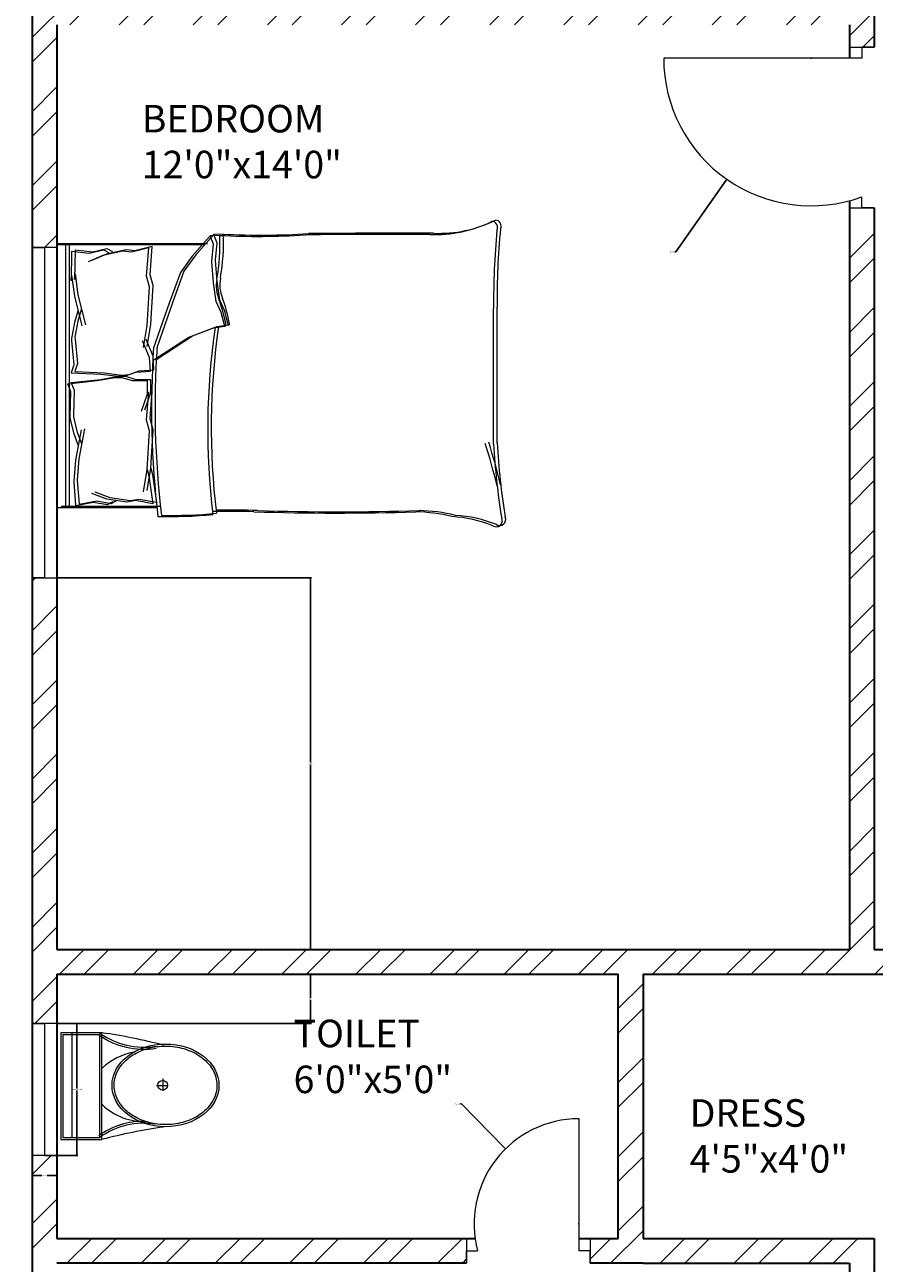
# Model space of a CAD drawing. Units: inches. Extents: x 392 to 1254, y 1207 to 2665.
# Tile 6 of 15: x 540 to 694, y 1827 to 2052. Entities that reach past the tile are written whole.
import ezdxf

# ---------------------------------------------------------------- set-up
doc = ezdxf.new("R2010")
doc.units = ezdxf.units.IN
for name, color, linetype, lineweight in [('A-ANNO-DIMS', 2, 'Continuous', 18), ('A-AREA-IDEN', 7, 'Continuous', 18), ('A-DOOR', 3, 'Continuous', 18), ('A-FLOR-FIXT', 9, 'Continuous', 18), ('A-FURN', 8, 'Continuous', 13), ('A-GLAZ', 4, 'Continuous', 18), ('A-WALL', 7, 'Continuous', 35), ('A-WALL-PATT', 252, 'Continuous', 13)]:
    doc.layers.add(name, color=color, linetype=linetype, lineweight=lineweight)
doc.styles.get("Standard").update_dxf_attribs({"font": 'arial.ttf'})
doc.dimstyles.get("Standard").update_dxf_attribs({"dimtxt": 0.18, "dimasz": 0.18, "dimexe": 0.18, "dimexo": 0.0625, "dimgap": 0.09, "dimtad": 0, "dimtih": 1, "dimtoh": 1, "dimdec": 4, "dimzin": 0, "dimdsep": 46, "dimtxsty": 'Standard', "dimcen": 0.09, "dimadec": 0, "dimazin": 0, "dimtfac": 1, "dimtdec": 4, "dimtofl": 0, "dimtmove": 0, "dimatfit": 3, "dimfxl": 1, "dimtolj": 1, "dimtzin": 0, "dimarcsym": 0})

# ---------------------------------------------------------------- blocks, each defined once
blk = doc.blocks.new('A$C31115884')
for p, q in [((283.1, 497.7), (223.4, 497.7)), ((257.5, 466.4), (257.5, 523.2)), ((0, 200), (0, 0)), ((520, 200), (0, 200)), ((10, 190), (10, 10)), ((510, 190), (10, 190)), ((510, 10), (510, 190)), ((520, 0), (520, 200)), ((510, 54.5), (0, 54.5)), ((10, 10), (510, 10)), ((0, 0), (520, 0))]:
    blk.add_line(p, q)
blk.add_circle((255.6, 496.4), 23.6)
for centre, radius, start, end in [((2777.7, -204.6), 2807, 165.4549, 171.71327), ((3237, 905), 2807, 188.28673, 194.5451), ((-294.5, 403.3), 364.7, 324.20913, 9.34987), ((-294.5, 403.3), 374.7, 324.20913, 9.34987), ((805.8, 403.3), 364.7, 170.65013, 215.79087), ((139.5, 406.2), 293.5, 315.84364, 2.65635), ((805.8, 403.3), 374.7, 179.20365, 215.79087), ((383.6, 406.2), 293.5, 190.27735, 224.15636)]:
    blk.add_arc(centre, radius, start, end)
blk.add_ellipse((256.2, 509.9), major_axis=(0, -260.7), ratio=0.772727)
blk.add_open_spline([(256.2, 259.2), (263.1, 259.2), (270, 259.7), (287.8, 262.3), (298.7, 265.1), (319.9, 273.1), (330.2, 278.4), (350.1, 291.1), (359.7, 298.7), (377.7, 315.9), (386.2, 325.5), (401.7, 346.6), (408.8, 358.1), (421.3, 382.5), (426.8, 395.5), (435.9, 422.4), (439.5, 436.4), (444.8, 465.1), (446.5, 479.7), (447.9, 509.2), (447.6, 524), (445, 553.3), (442.7, 567.8), (436.3, 596), (432.1, 609.7), (421.9, 636), (416, 648.6), (402.5, 672.1), (395, 683), (378.6, 703), (369.8, 712.1), (351.1, 728), (341.3, 734.8), (320.9, 746.2), (310.4, 750.7), (288.9, 757.3), (278, 759.4), (256, 761), (245, 760.6), (223.1, 757.2), (212.3, 754.3), (191.1, 746.1), (180.8, 740.7), (160.9, 727.8), (151.4, 720.1), (133.5, 702.7), (125.1, 693), (109.6, 671.7), (102.6, 660.2), (90.2, 635.7), (84.9, 622.7), (76, 595.6), (72.4, 581.6), (67.2, 552.9), (65.6, 538.2), (64.4, 508.8), (64.8, 494), (67.5, 464.7), (69.9, 450.2), (76.6, 422), (80.8, 408.3), (91.1, 382.2), (97.2, 369.7), (110.8, 346.3), (118.4, 335.4), (134.8, 315.6), (143.7, 306.7), (162.4, 290.9), (172.3, 284.2), (192.8, 273), (203.3, 268.6), (224.8, 262.2), (235.8, 260.2), (249.9, 259.3), (253, 259.2), (256.2, 259.2)], degree=3, knots=[0, 0, 0, 0, 0.110105, 0.110105, 0.285049, 0.285049, 0.459994, 0.459994, 0.634938, 0.634938, 0.809882, 0.809882, 0.984827, 0.984827, 1.159771, 1.159771, 1.334715, 1.334715, 1.50966, 1.50966, 1.684604, 1.684604, 1.859549, 1.859549, 2.034493, 2.034493, 2.209437, 2.209437, 2.384382, 2.384382, 2.559326, 2.559326, 2.73427, 2.73427, 2.909215, 2.909215, 3.084159, 3.084159, 3.259103, 3.259103, 3.434048, 3.434048, 3.608992, 3.608992, 3.783936, 3.783936, 3.958881, 3.958881, 4.133825, 4.133825, 4.30877, 4.30877, 4.483714, 4.483714, 4.658658, 4.658658, 4.833603, 4.833603, 5.008547, 5.008547, 5.183491, 5.183491, 5.358436, 5.358436, 5.53338, 5.53338, 5.708324, 5.708324, 5.883269, 5.883269, 6.058213, 6.058213, 6.233158, 6.233158, 6.283185, 6.283185, 6.283185, 6.283185])
blk = doc.blocks.new('BED-DOUBLE')
for p, q in [((3.47, 63.33), (3.47, 81.44)), ((3.48, 63.33), (3.48, 81.44)), ((51.27, 81.44), (51.27, 54.83)), ((51.27, 81.44), (51.27, 54.83)), ((51.49, 81.44), (51.49, 80.8)), ((3.47, 79.91), (51.27, 79.91)), ((3.48, 79.91), (51.27, 79.91)), ((3.7, 62.69), (3.7, 80.8)), ((3.7, 62.69), (3.7, 80.8)), ((3.7, 79.27), (51.49, 79.27)), ((3.7, 79.27), (51.49, 79.27)), ((16.88, 78.42), (19.77, 79.14)), ((16.88, 78.42), (19.77, 79.14)), ((19.77, 79.14), (20.09, 79.14)), ((19.77, 79.14), (20.09, 79.14)), ((20.09, 79.14), (24.54, 78.99)), ((20.09, 79.14), (24.54, 78.99)), ((24.54, 78.99), (25.98, 79.57)), ((24.54, 78.99), (25.98, 79.57)), ((24.77, 78.35), (26.21, 78.93)), ((24.77, 78.35), (26.21, 78.93)), ((25.98, 79.57), (26.56, 74.22)), ((25.98, 79.57), (26.56, 74.22)), ((26.21, 78.93), (26.79, 73.58)), ((26.21, 78.93), (26.79, 73.58)), ((27.98, 78.95), (27.73, 73.58)), ((27.98, 78.95), (27.73, 73.58)), ((29.46, 78.46), (27.98, 78.95)), ((29.46, 78.46), (27.98, 78.95)), ((33.88, 78.89), (29.46, 78.46)), ((33.88, 78.89), (29.46, 78.46)), ((34.2, 78.91), (33.88, 78.89)), ((34.2, 78.91), (33.88, 78.89)), ((37.14, 78.36), (34.2, 78.91)), ((37.14, 78.36), (34.2, 78.91)), ((45.71, 78.9), (41.91, 78.37)), ((45.71, 78.9), (41.91, 78.37)), ((50.11, 78.89), (44.71, 78.98)), ((44.71, 78.98), (45.71, 78.9)), ((50.11, 78.89), (44.71, 78.98)), ((44.71, 78.98), (45.71, 78.9)), ((50.11, 78.89), (49.73, 75.67)), ((50.11, 78.89), (49.73, 75.67)), ((51.49, 80.8), (51.49, 54.19)), ((51.49, 80.8), (51.49, 54.19)), ((3.89, 78.13), (4.47, 74.95)), ((3.89, 78.13), (4.47, 74.95)), ((3.9, 78.1), (8.18, 78.43)), ((3.9, 78.1), (8.18, 78.43)), ((4.12, 77.49), (4.7, 74.31)), ((4.12, 77.49), (4.7, 74.31)), ((4.13, 77.47), (8.41, 77.79)), ((4.13, 77.47), (8.41, 77.79)), ((8.18, 78.43), (8.28, 78.42)), ((8.18, 78.43), (8.28, 78.42)), ((8.28, 78.42), (12.11, 78.13)), ((8.28, 78.42), (12.11, 78.13)), ((8.41, 77.79), (8.51, 77.78)), ((8.41, 77.79), (8.51, 77.78)), ((8.51, 77.78), (12.34, 77.49)), ((8.51, 77.78), (12.34, 77.49)), ((12.11, 78.13), (17.6, 77.11)), ((12.11, 78.13), (17.6, 77.11)), ((12.34, 77.49), (17.83, 76.48)), ((12.34, 77.49), (17.83, 76.48)), ((14.85, 77.69), (16.88, 78.42)), ((14.85, 77.69), (16.88, 78.42)), ((15.08, 77.05), (17.11, 77.78)), ((15.08, 77.05), (17.11, 77.78)), ((17.11, 77.78), (20, 78.5)), ((17.11, 77.78), (20, 78.5)), ((20, 78.5), (20.32, 78.5)), ((20, 78.5), (20.32, 78.5)), ((20.32, 78.5), (24.77, 78.35)), ((20.32, 78.5), (24.77, 78.35)), ((28.21, 78.31), (27.96, 72.94)), ((28.21, 78.31), (27.96, 72.94)), ((29.68, 77.82), (28.21, 78.31)), ((29.68, 77.82), (28.21, 78.31)), ((34.11, 78.25), (29.68, 77.82)), ((34.11, 78.25), (29.68, 77.82)), ((34.43, 78.27), (34.11, 78.25)), ((34.43, 78.27), (34.11, 78.25)), ((37.36, 77.73), (34.43, 78.27)), ((37.36, 77.73), (34.43, 78.27)), ((41.91, 78.37), (36.49, 77.02)), ((41.91, 78.37), (36.5, 77.02)), ((42.14, 77.73), (36.72, 76.38)), ((42.14, 77.73), (36.72, 76.38)), ((39.2, 77.77), (37.14, 78.36)), ((39.2, 77.77), (37.14, 78.36)), ((39.43, 77.13), (37.36, 77.73)), ((39.43, 77.13), (37.36, 77.73)), ((45.94, 78.26), (42.14, 77.73)), ((45.94, 78.26), (42.14, 77.73)), ((50.34, 78.25), (44.94, 78.34)), ((44.94, 78.34), (45.94, 78.26)), ((50.34, 78.25), (44.94, 78.34)), ((44.94, 78.34), (45.94, 78.26)), ((50.34, 78.25), (49.96, 75.04)), ((50.34, 78.25), (49.96, 75.04)), ((4.47, 74.95), (4.04, 72.34)), ((4.47, 74.95), (4.04, 72.34)), ((4.7, 74.31), (4.27, 71.7)), ((4.7, 74.31), (4.27, 71.7)), ((5.05, 72.49), (6.06, 75.23)), ((5.05, 72.49), (6.06, 75.23)), ((5.28, 71.85), (6.29, 74.6)), ((5.28, 71.85), (6.29, 74.6)), ((49.31, 73.19), (48.13, 75.86)), ((49.31, 73.19), (48.13, 75.86)), ((49.54, 72.55), (48.36, 75.22)), ((49.54, 72.55), (48.36, 75.22)), ((49.73, 75.67), (50.33, 73.1)), ((49.73, 75.67), (50.33, 73.1)), ((49.96, 75.04), (50.56, 72.47)), ((49.96, 75.04), (50.56, 72.47)), ((4.04, 72.34), (4.62, 71.33)), ((4.04, 72.34), (4.62, 71.33)), ((4.47, 68.87), (5.05, 72.49)), ((4.47, 68.87), (5.05, 72.49)), ((26.56, 74.22), (27.14, 71.04)), ((26.56, 74.22), (27.14, 71.04)), ((26.79, 73.58), (27.37, 70.4)), ((26.79, 73.58), (27.37, 70.4)), ((27.73, 73.58), (27.35, 70.36)), ((27.73, 73.58), (27.35, 70.36)), ((27.96, 72.94), (27.58, 69.73)), ((27.96, 72.94), (27.58, 69.73)), ((50.11, 69.61), (49.31, 73.19)), ((50.11, 69.61), (49.31, 73.19)), ((50.34, 68.97), (49.54, 72.55)), ((50.34, 68.97), (49.54, 72.55)), ((50.33, 73.1), (49.81, 72.06)), ((50.33, 73.1), (49.81, 72.06)), ((50.56, 72.47), (50.04, 71.42)), ((50.56, 72.47), (50.04, 71.42)), ((4.27, 71.7), (4.85, 70.69)), ((4.27, 71.7), (4.85, 70.69)), ((4.7, 68.23), (5.28, 71.85)), ((4.7, 68.23), (5.28, 71.85)), ((27.14, 71.04), (27.14, 69.74)), ((27.14, 71.04), (27.14, 69.74)), ((27.35, 70.36), (27.44, 69.07)), ((27.35, 70.36), (27.44, 69.07)), ((27.37, 70.4), (27.37, 69.1)), ((27.37, 70.4), (27.37, 69.1)), ((4.76, 67.28), (4.47, 68.87)), ((4.76, 67.28), (4.47, 68.87)), ((4.99, 66.64), (4.7, 68.23)), ((4.99, 66.64), (4.7, 68.23)), ((27.14, 69.74), (26.56, 67.86)), ((27.14, 69.74), (26.56, 67.86)), ((26.56, 67.86), (26.56, 65.18)), ((26.56, 67.86), (26.56, 65.18)), ((27.37, 69.1), (26.79, 67.22)), ((27.37, 69.1), (26.79, 67.22)), ((27.44, 69.07), (28.13, 67.23)), ((27.44, 69.07), (28.13, 67.23)), ((27.58, 69.73), (27.66, 68.43)), ((27.58, 69.73), (27.66, 68.43)), ((27.66, 68.43), (28.36, 66.59)), ((27.66, 68.43), (28.36, 66.59)), ((49.92, 68.01), (50.11, 69.61)), ((49.92, 68.01), (50.11, 69.61)), ((50.7, 64.87), (49.92, 68.01)), ((50.7, 64.87), (49.92, 68.01)), ((50.15, 67.37), (50.34, 68.97)), ((50.15, 67.37), (50.34, 68.97)), ((4.18, 64.1), (4.76, 67.28)), ((4.18, 64.1), (4.76, 67.28)), ((4.41, 63.46), (4.99, 66.64)), ((4.41, 63.46), (4.99, 66.64)), ((6.38, 65.81), (10.41, 65.15)), ((6.38, 65.81), (10.41, 65.15)), ((17.42, 64.72), (19.38, 65.27)), ((17.42, 64.72), (19.38, 65.27)), ((19.38, 65.27), (24.52, 64.87)), ((19.38, 65.27), (24.52, 64.87)), ((24.1, 65.18), (20.96, 66.27)), ((24.1, 65.18), (20.96, 66.27)), ((24.33, 64.54), (21.19, 65.63)), ((24.33, 64.54), (21.19, 65.63)), ((26.79, 67.22), (26.79, 64.54)), ((26.79, 67.22), (26.79, 64.54)), ((28.13, 67.23), (28.3, 64.55)), ((28.13, 67.23), (28.3, 64.55)), ((28.36, 66.59), (28.53, 63.91)), ((28.36, 66.59), (28.53, 63.91)), ((30.75, 64.7), (33.82, 65.99)), ((30.75, 64.7), (33.82, 65.99)), ((30.98, 64.06), (34.05, 65.35)), ((30.98, 64.06), (34.05, 65.35)), ((32.56, 65.81), (36.6, 65.15)), ((32.56, 65.81), (36.6, 65.15)), ((43.61, 64.72), (45.57, 65.27)), ((43.61, 64.72), (45.57, 65.27)), ((45.57, 65.27), (50.7, 64.87)), ((45.57, 65.27), (50.7, 64.87)), ((50.93, 64.23), (50.15, 67.37)), ((50.93, 64.23), (50.15, 67.37)), ((9.28, 64.82), (4.18, 64.1)), ((9.28, 64.82), (4.18, 64.1)), ((9.51, 64.19), (4.41, 63.46)), ((9.51, 64.19), (4.41, 63.46)), ((6.61, 65.17), (10.64, 64.51)), ((6.61, 65.17), (10.64, 64.51)), ((10.41, 65.15), (9.28, 64.82)), ((10.41, 65.15), (9.28, 64.82)), ((10.64, 64.51), (9.51, 64.19)), ((10.64, 64.51), (9.51, 64.19)), ((10.41, 65.15), (17.42, 64.72)), ((10.41, 65.15), (17.42, 64.72)), ((10.64, 64.51), (17.65, 64.08)), ((10.64, 64.51), (17.65, 64.08)), ((17.65, 64.08), (19.61, 64.63)), ((17.65, 64.08), (19.61, 64.63)), ((19.61, 64.63), (24.74, 64.23)), ((19.61, 64.63), (24.74, 64.23)), ((26.56, 65.18), (24.1, 65.18)), ((26.56, 65.18), (24.1, 65.18)), ((26.79, 64.54), (24.33, 64.54)), ((26.79, 64.54), (24.33, 64.54)), ((28.3, 64.55), (30.75, 64.7)), ((28.3, 64.55), (30.75, 64.7)), ((28.53, 63.91), (30.98, 64.06)), ((28.53, 63.91), (30.98, 64.06)), ((30.26, 64.06), (34.45, 57.57)), ((30.26, 64.06), (34.45, 57.57)), ((30.49, 63.42), (34.68, 56.93)), ((30.49, 63.42), (34.68, 56.93)), ((40.64, 61.13), (32.31, 64.06)), ((40.64, 61.13), (32.31, 64.06)), ((40.87, 60.49), (32.53, 63.42)), ((40.87, 60.49), (32.53, 63.42)), ((32.79, 65.17), (36.82, 64.51)), ((32.79, 65.17), (36.82, 64.51)), ((36.6, 65.15), (43.61, 64.72)), ((36.6, 65.15), (43.61, 64.72)), ((36.82, 64.51), (43.83, 64.08)), ((36.82, 64.51), (43.83, 64.08)), ((43.83, 64.08), (45.79, 64.63)), ((43.83, 64.08), (45.79, 64.63)), ((45.79, 64.63), (50.93, 64.23)), ((45.79, 64.63), (50.93, 64.23)), ((46.22, 59.11), (40.64, 61.13)), ((46.22, 59.11), (40.64, 61.13)), ((46.45, 58.47), (40.87, 60.49)), ((46.45, 58.47), (40.87, 60.49)), ((49.16, 56.95), (46.22, 59.11)), ((49.16, 56.95), (46.22, 59.11)), ((34.45, 57.57), (36.15, 53.08)), ((34.45, 57.57), (36.15, 53.08)), ((34.68, 56.93), (36.38, 52.44)), ((34.68, 56.93), (36.38, 52.44)), ((49.39, 56.31), (46.45, 58.47)), ((49.39, 56.31), (46.45, 58.47)), ((52.87, 53.7), (49.16, 56.95)), ((52.87, 53.7), (49.16, 56.95)), ((53.1, 53.06), (49.39, 56.31)), ((53.1, 53.06), (49.39, 56.31)), ((36.15, 53.08), (36.46, 51.07)), ((36.15, 53.08), (36.46, 51.07)), ((36.38, 52.44), (36.69, 50.43)), ((36.38, 52.44), (36.69, 50.43)), ((38.94, 51.68), (40.95, 52.61)), ((38.94, 51.68), (40.95, 52.61)), ((39.17, 51.05), (41.18, 51.97)), ((39.17, 51.05), (41.18, 51.97)), ((40.95, 52.61), (44.36, 53.08)), ((40.95, 52.61), (44.36, 53.08)), ((41.18, 51.97), (44.59, 52.44)), ((41.18, 51.97), (44.59, 52.44)), ((44.36, 53.08), (48.23, 53.39)), ((44.36, 53.08), (48.23, 53.39)), ((44.59, 52.44), (48.46, 52.75)), ((44.59, 52.44), (48.46, 52.75)), ((48.23, 53.39), (51.33, 53.08)), ((48.23, 53.39), (51.33, 53.08)), ((48.46, 52.75), (51.56, 52.44)), ((48.46, 52.75), (51.56, 52.44)), ((51.33, 53.08), (52.87, 53.7)), ((51.33, 53.08), (52.87, 53.7)), ((51.56, 52.44), (53.1, 53.06)), ((51.56, 52.44), (53.1, 53.06)), ((52.95, 51.95), (52.87, 53.7, 3.87)), ((52.95, 51.95), (52.87, 53.7, 3.87)), ((53.18, 51.31), (53.1, 53.06, 3.87)), ((53.18, 51.31), (53.1, 53.06, 3.87)), ((36.46, 51.07), (38.94, 51.68)), ((36.46, 51.07), (38.94, 51.68)), ((36.69, 50.43), (39.17, 51.05)), ((36.69, 50.43), (39.17, 51.05)), ((15.06, 2.2), (39.68, 2.2)), ((15.06, 2.2), (39.68, 2.2)), ((15.29, 1.56), (39.91, 1.56)), ((15.29, 1.56), (39.91, 1.56))]:
    blk.add_line(p, q)
for centre, radius, start, end in [((85.16, 61.35), 83.31, 178.7218, 185.604), ((85.16, 61.35), 83.31, 178.7218, 185.604), ((21.36, -100.61), 164.97, 86.0865, 96.7821), ((21.36, -100.61), 164.97, 86.0865, 96.7821), ((21.59, -101.25), 164.97, 86.0865, 96.7821), ((21.59, -101.25), 164.97, 86.0865, 96.7821), ((85.39, 60.71), 83.31, 178.7218, 185.604), ((85.39, 60.71), 83.31, 178.7218, 185.604), ((17.76, -74.87), 129.02, 81.7845, 96.9006), ((17.76, -74.87), 129.02, 81.7845, 96.9006), ((17.98, -75.51), 129.02, 81.7845, 96.9006), ((17.98, -75.51), 129.02, 81.7845, 96.9006), ((-167.31, 50.27), 170.11, 358.4762, 1.0082), ((-167.31, 50.27), 170.11, 358.4762, 1.0082), ((-167.08, 49.63), 170.11, 358.4762, 1.0082), ((-167.08, 49.63), 170.11, 358.4762, 1.0082), ((31.15, 79.96), 29.65, 280.6617, 289.8806), ((31.15, 79.96), 29.65, 280.6617, 289.8806), ((43.74, 46.38), 6.22, 78.6608, 113.7384), ((43.74, 46.38), 6.22, 78.6608, 113.7384), ((43.97, 45.74), 6.22, 78.6608, 113.7384), ((43.97, 45.74), 6.22, 78.6608, 113.7384), ((51.33, 88.1), 36.18, 259.8763, 272.5657), ((51.33, 88.1), 36.18, 259.8763, 272.5657), ((51.56, 87.46), 36.18, 259.8763, 272.5657), ((51.56, 87.46), 36.18, 259.8763, 272.5657), ((182.27, 45.13), 129.5, 176.9791, 183.8365), ((182.27, 45.13), 129.5, 176.9791, 183.8365), ((36.64, 51), 0.185, 160.2464, 271.1377), ((36.64, 51), 0.185, 160.2464, 271.1377), ((36.86, 50.36), 0.185, 160.2464, 271.1377), ((36.86, 50.36), 0.185, 160.2464, 271.1377), ((31.38, 79.32), 29.65, 280.6617, 289.8806), ((31.38, 79.32), 29.65, 280.6617, 289.8806), ((182.49, 44.49), 129.5, 176.9791, 183.8365), ((182.49, 44.49), 129.5, 176.9791, 183.8365), ((484.82, 30.83), 482.31, 178.2277, 181.7185), ((484.82, 30.83), 482.31, 178.2277, 181.7185), ((485.05, 30.19), 482.31, 178.2277, 181.7185), ((485.05, 30.19), 482.31, 178.2277, 181.7185), ((-4508.74, 13.62), 4561.86, 0.00217, 0.28689), ((-4508.74, 13.62), 4561.86, 0.00217, 0.28689), ((-4508.51, 12.98), 4561.86, 0.00217, 0.28689), ((-4508.52, 12.98), 4561.86, 0.00217, 0.28689), ((-26.9, 16.93), 29.63, 346.0648, 358.9113), ((-26.9, 16.93), 29.63, 346.0648, 358.9113), ((-26.67, 16.29), 29.63, 346.0648, 358.9113), ((-26.67, 16.29), 29.63, 346.0648, 358.9113), ((76.16, 12.78), 23.07, 177.4714, 206.4681), ((76.16, 12.78), 23.07, 177.4714, 206.4681), ((76.39, 12.14), 23.07, 177.4714, 206.4681), ((76.39, 12.14), 23.07, 177.4714, 206.4681), ((-21.66, 11.17), 23.56, 337.9751, 356.652), ((-21.66, 11.17), 23.56, 337.9751, 356.652), ((-21.43, 10.53), 23.56, 337.9751, 356.652), ((-21.43, 10.53), 23.56, 337.9751, 356.652), ((1.09, 1.72), 1.09, 146.1736, 293.4781), ((1.09, 1.72), 1.09, 146.1736, 293.4781), ((-17.22, 105.15), 106.46, 283.3832, 287.7053), ((-17.22, 105.15), 106.46, 283.3832, 287.7053), ((-16.99, 104.52), 106.46, 283.3832, 287.7053), ((-16.99, 104.52), 106.46, 283.3832, 287.7053), ((54.41, 2.57), 1.1, 242.6588, 356.02), ((54.41, 2.57), 1.1, 242.6588, 356.02), ((1.32, 1.09), 1.09, 146.1736, 293.4781), ((1.32, 1.09), 1.09, 146.1736, 293.4781), ((21.43, -119.39), 121.76, 92.9958, 99.4091), ((21.43, -119.39), 121.76, 92.9958, 99.4091), ((21.66, -120.03), 121.76, 92.9958, 99.4091), ((21.65, -120.03), 121.76, 92.9958, 99.4091), ((41.15, -130.83), 133.04, 84.4998, 90.6351), ((41.15, -130.83), 133.04, 84.4998, 90.6351), ((41.38, -131.47), 133.04, 84.4998, 90.6351), ((41.38, -131.47), 133.04, 84.4998, 90.6351), ((54.64, 1.93), 1.1, 242.6588, 356.02), ((54.64, 1.93), 1.1, 242.6588, 356.02)]:
    blk.add_arc(centre, radius, start, end)
blk = doc.blocks.new('WIN-24-B')
for p, q in [((2.25, 24), (0, 24)), ((0, 24), (4.5, 24)), ((2.25, 0), (2.25, 24)), ((0, 0), (4.5, 0)), ((4.5, 0), (2.25, 0))]:
    blk.add_line(p, q)
blk = doc.blocks.new('WIN-60-B')
for p, q in [((4.5, 60), (0, 60)), ((2.25, 0), (2.25, 60)), ((2.25, 60), (4.5, 60)), ((0, 0), (4.5, 0)), ((4.5, 0), (2.25, 0))]:
    blk.add_line(p, q)
blk = doc.blocks.new('*D17')
at = {"layer": 'A-ANNO-DIMS', "color": 0, "lineweight": -2, "transparency": 16777216}
for p, q in [((545.84, 1870.85), (549.56, 1870.85)), ((549.38, 1870.67), (549.38, 1859.03)), ((549.38, 1847.03), (549.38, 1858.67)), ((545.84, 1846.85), (549.56, 1846.85))]:
    blk.add_line(p, q, dxfattribs=at)
at = {"layer": 'A-ANNO-DIMS', "color": 0, "transparency": 16777216}
for points in [[(549.35, 1870.67), (549.41, 1870.67), (549.38, 1870.85)], [(549.35, 1847.03), (549.41, 1847.03), (549.38, 1846.85)]]:
    blk.add_solid(points, dxfattribs=at)
at = {"layer": 'Defpoints', "color": 0, "transparency": 16777216}
for p in [(545.78, 1870.85), (545.78, 1846.85), (549.38, 1846.85)]:
    blk.add_point(p, dxfattribs=at)
at = {"layer": 'A-ANNO-DIMS', "color": 0, "transparency": 16777216, "insert": (549.38, 1858.85), "char_height": 0.18, "attachment_point": 5}
blk.add_mtext('\\A1;WINDOW B 24 TYP.', dxfattribs=at)
blk = doc.blocks.new('*D18')
at = {"layer": 'A-ANNO-DIMS', "color": 0, "lineweight": -2, "transparency": 16777216}
for p, q in [((541.28, 1846.79), (541.28, 1843.07)), ((545.78, 1846.79), (545.78, 1843.07)), ((541.46, 1843.25), (543.07, 1843.25)), ((545.6, 1843.25), (543.99, 1843.25))]:
    blk.add_line(p, q, dxfattribs=at)
at = {"layer": 'A-ANNO-DIMS', "color": 0, "transparency": 16777216}
for points in [[(541.46, 1843.28), (541.46, 1843.22), (541.28, 1843.25)], [(545.6, 1843.28), (545.6, 1843.22), (545.78, 1843.25)]]:
    blk.add_solid(points, dxfattribs=at)
at = {"layer": 'Defpoints', "color": 0, "transparency": 16777216}
for p in [(541.28, 1846.85), (545.78, 1846.85), (541.28, 1843.25)]:
    blk.add_point(p, dxfattribs=at)
at = {"layer": 'A-ANNO-DIMS', "color": 0, "transparency": 16777216, "insert": (543.53, 1843.25), "char_height": 0.18, "attachment_point": 5}
blk.add_mtext('\\A1;5 TYP.', dxfattribs=at)
blk = doc.blocks.new('*D26')
at = {"layer": 'A-ANNO-DIMS', "color": 0, "lineweight": -2, "transparency": 16777216}
for p, q in [((541.22, 2229.3), (495, 2229.3)), ((495.18, 2229.12), (495.18, 1819.98)), ((495.18, 1410.48), (495.18, 1819.61)), ((753.23, 1410.3), (495, 1410.3))]:
    blk.add_line(p, q, dxfattribs=at)
at = {"layer": 'A-ANNO-DIMS', "color": 0, "transparency": 16777216}
for points in [[(495.15, 2229.12), (495.21, 2229.12), (495.18, 2229.3)], [(495.15, 1410.48), (495.21, 1410.48), (495.18, 1410.3)]]:
    blk.add_solid(points, dxfattribs=at)
at = {"layer": 'Defpoints', "color": 0, "transparency": 16777216}
for p in [(495.18, 2229.3), (541.28, 2229.3), (753.29, 1410.3)]:
    blk.add_point(p, dxfattribs=at)
at = {"layer": 'A-ANNO-DIMS', "color": 0, "transparency": 16777216, "insert": (495.18, 1819.8), "char_height": 0.18, "attachment_point": 5}
blk.add_mtext('\\A1;819', dxfattribs=at)
blk = doc.blocks.new('*D36')
at = {"layer": 'A-ANNO-DIMS', "color": 0, "lineweight": -2, "transparency": 16777216}
for p, q in [((545.84, 1951.82), (592.06, 1951.82)), ((591.88, 1951.64), (591.88, 1918.24)), ((591.88, 1884.48), (591.88, 1917.88)), ((545.84, 1884.3), (592.06, 1884.3))]:
    blk.add_line(p, q, dxfattribs=at)
at = {"layer": 'A-ANNO-DIMS', "color": 0, "transparency": 16777216}
for points in [[(591.85, 1951.64), (591.91, 1951.64), (591.88, 1951.82)], [(591.85, 1884.48), (591.91, 1884.48), (591.88, 1884.3)]]:
    blk.add_solid(points, dxfattribs=at)
at = {"layer": 'Defpoints', "color": 0, "transparency": 16777216}
for p in [(545.78, 1951.82), (545.78, 1884.3), (591.88, 1884.3)]:
    blk.add_point(p, dxfattribs=at)
at = {"layer": 'A-ANNO-DIMS', "color": 0, "transparency": 16777216, "insert": (591.88, 1918.06), "char_height": 0.18, "attachment_point": 5}
blk.add_mtext('\\A1;67.53', dxfattribs=at)
blk = doc.blocks.new('*D37')
at = {"layer": 'A-ANNO-DIMS', "color": 0, "lineweight": -2, "transparency": 16777216}
for p, q in [((545.84, 1879.8), (592.06, 1879.8)), ((591.88, 1879.62), (591.88, 1875.51)), ((591.88, 1871.03), (591.88, 1875.14)), ((545.84, 1870.85), (592.06, 1870.85))]:
    blk.add_line(p, q, dxfattribs=at)
at = {"layer": 'A-ANNO-DIMS', "color": 0, "transparency": 16777216}
for points in [[(591.85, 1879.62), (591.91, 1879.62), (591.88, 1879.8)], [(591.85, 1871.03), (591.91, 1871.03), (591.88, 1870.85)]]:
    blk.add_solid(points, dxfattribs=at)
at = {"layer": 'Defpoints', "color": 0, "transparency": 16777216}
for p in [(545.78, 1879.8), (545.78, 1870.85), (591.88, 1870.85)]:
    blk.add_point(p, dxfattribs=at)
at = {"layer": 'A-ANNO-DIMS', "color": 0, "transparency": 16777216, "insert": (591.88, 1875.32), "char_height": 0.18, "attachment_point": 5}
blk.add_mtext('\\A1;8.944', dxfattribs=at)
blk = doc.blocks.new('*D93')
at = {"layer": 'A-ANNO-DIMS', "color": 0, "lineweight": -2, "transparency": 16777216}
for p, q in [((682.74, 2046.2), (682.92, 2046.2)), ((682.83, 2046.11), (682.83, 2046.29)), ((658.26, 2011.06), (667.37, 2024.09)), ((658.08, 2011.06), (658.26, 2011.06))]:
    blk.add_line(p, q, dxfattribs=at)
at = {"layer": 'A-ANNO-DIMS', "color": 0, "transparency": 16777216}
blk.add_solid([(667.35, 2024.11), (667.39, 2024.08), (667.47, 2024.24)], dxfattribs=at)
at = {"layer": 'Defpoints', "color": 0, "transparency": 16777216}
for p in [(682.83, 2046.2), (667.47, 2024.24)]:
    blk.add_point(p, dxfattribs=at)
at = {"layer": 'A-ANNO-DIMS', "color": 0, "transparency": 16777216, "insert": (657.53, 2011.06), "char_height": 0.18, "attachment_point": 5}
blk.add_mtext('\\A1;R26.803', dxfattribs=at)
blk = doc.blocks.new('*D101')
at = {"layer": 'A-ANNO-DIMS', "color": 0, "lineweight": -2, "transparency": 16777216}
for p, q in [((619.12, 1856.27), (619.3, 1856.27)), ((619.3, 1856.27), (627.18, 1848.23)), ((640.55, 1834.48), (640.73, 1834.48)), ((640.64, 1834.39), (640.64, 1834.57))]:
    blk.add_line(p, q, dxfattribs=at)
at = {"layer": 'A-ANNO-DIMS', "color": 0, "transparency": 16777216}
blk.add_solid([(627.2, 1848.25), (627.15, 1848.21), (627.3, 1848.1)], dxfattribs=at)
at = {"layer": 'Defpoints', "color": 0, "transparency": 16777216}
for p in [(627.3, 1848.1), (640.64, 1834.48)]:
    blk.add_point(p, dxfattribs=at)
at = {"layer": 'A-ANNO-DIMS', "color": 0, "transparency": 16777216, "insert": (618.57, 1856.27), "char_height": 0.18, "attachment_point": 5}
blk.add_mtext('\\A1;R19.066', dxfattribs=at)

msp = doc.modelspace()

# ---------------------------------------------------------------- hatches: boundary and pattern name
at = {"layer": 'A-WALL-PATT'}
h = msp.add_hatch(dxfattribs=at)
h.set_pattern_fill('ANSI32', color=256)
h.paths.add_polyline_path([(579.5309, 2227.0453), (579.5309, 2229.2953), (541.2807, 2229.2953), (541.2807, 2182.3091), (545.7807, 2182.3091), (545.7807, 2224.7953), (579.5309, 2224.7953)])
h.paths.add_polyline_path([(655.4442, 2229.2953), (627.5309, 2229.2953), (627.5309, 2224.7953), (655.4442, 2224.7953), (655.4442, 2227.0453)])
h.paths.add_polyline_path([(703.0758, 2229.2953), (678.5257, 2229.2953), (678.5257, 2227.0453), (678.5257, 2224.7953), (689.7807, 2224.7953), (689.7807, 2158.6973), (694.2807, 2158.6973), (694.2807, 2224.7953), (703.0758, 2224.7953)])
h.paths.add_polyline_path([(768.5767, 2229.2953), (727.0758, 2229.2953), (727.0758, 2224.7953), (742.2807, 2224.7953), (742.2807, 2128.7953), (694.2807, 2128.7953), (694.2807, 2134.0554), (689.7807, 2134.0554), (689.7807, 2090.2854), (694.2807, 2090.2854), (694.2807, 2124.2953), (742.2807, 2124.2953), (742.2807, 2052.2953), (795.2124, 2052.2953), (795.2124, 2054.5453), (795.2124, 2056.7953), (746.7807, 2056.7953), (746.7807, 2224.7953), (768.5767, 2224.7953)])
h.paths.add_polyline_path([(867.5089, 2229.2953), (804.5767, 2229.2953), (804.5767, 2224.7953), (830.7807, 2224.7953), (830.7807, 2056.7953), (826.9066, 2056.7953), (826.9066, 2052.2953), (830.7807, 2052.2953), (830.7807, 1886.6777, -0.01766664), (830.8602, 1884.2953), (835.0818, 1884.2953, -0.04411348), (835.2807, 1889.9369), (835.2807, 2052.2953), (839.418, 2052.2953), (839.418, 2056.7953), (835.2807, 2056.7953), (835.2807, 2224.7953), (867.5089, 2224.7953)])
h.paths.add_polyline_path([(939.8604, 2229.2953), (903.5089, 2229.2953), (903.5089, 2227.0453), (903.5089, 2224.7953), (919.2807, 2224.7953), (919.2807, 2056.7953), (870.6499, 2056.7953), (870.6499, 2052.2953), (923.7807, 2052.2953), (923.7807, 2124.2953), (971.7807, 2124.2953), (971.7807, 2089.7112), (974.0307, 2089.7112), (976.2807, 2089.7112), (976.2807, 2133.56), (974.0307, 2133.56), (971.7807, 2133.56), (971.7807, 2128.7953), (923.7807, 2128.7953), (923.7807, 2224.7953), (939.8604, 2224.7953)])
h.paths.add_polyline_path([(1124.7807, 2229.2953), (1009.403, 2229.2953), (1009.403, 2224.7953), (1120.2807, 2224.7953), (1120.2807, 2184.7605), (1124.7807, 2184.7605)])
h.paths.add_polyline_path([(1124.7807, 2124.7605), (1120.2807, 2124.7605), (1120.2807, 2056.7953), (976.2807, 2056.7953), (976.2807, 2061.471), (971.7807, 2061.471), (971.7807, 2047.7483), (974.0307, 2047.7483), (976.2807, 2047.7483), (976.2807, 2052.2953), (1120.2807, 2052.2953), (1120.2807, 1992.457), (1124.7807, 1992.457)])
h.paths.add_polyline_path([(1124.7807, 1932.457), (1122.5307, 1932.457), (1120.2807, 1932.457), (1120.2807, 1884.2953), (976.2807, 1884.2953), (976.2807, 2019.9536), (971.7807, 2019.9536), (971.7807, 1884.2953), (869.0911, 1884.2953), (869.0911, 1879.7953), (971.7807, 1879.7953), (1013.7807, 1879.7953), (1013.7807, 1831.7953), (971.7807, 1831.7953), (971.7807, 1822.3831), (974.0307, 1822.3831), (976.2807, 1822.3831), (976.2807, 1827.2953), (1013.7807, 1827.2953), (1025.6191, 1827.2953), (1025.6191, 1829.5453), (1025.6191, 1831.7953), (1018.2807, 1831.7953), (1018.2807, 1879.7953), (1120.2807, 1879.7953), (1120.2807, 1866.9192), (1124.7807, 1866.9192)])
h.paths.add_polyline_path([(1124.7807, 1842.9192), (1122.5307, 1842.9192), (1120.2807, 1842.9192), (1120.2807, 1831.7953), (1050.2021, 1831.7953), (1050.2021, 1827.2953), (1120.2807, 1827.2953), (1120.2807, 1781.4559), (1124.7807, 1781.4559)])
h.paths.add_polyline_path([(976.2807, 1790.8718), (971.7807, 1790.8718), (971.7807, 1648.3339), (976.2807, 1648.3339), (976.2807, 1654.7953), (1120.2807, 1654.7953), (1120.2807, 1626.3807), (1124.7807, 1626.3807), (1124.7807, 1721.4559), (1120.2807, 1721.4559), (1120.2807, 1659.2953), (976.2807, 1659.2953)])
h.paths.add_polyline_path([(1124.7807, 1566.3807), (1120.2807, 1566.3807), (1120.2807, 1486.7953), (1101.07, 1486.7953), (1101.07, 1482.2953), (1124.7807, 1482.2953)])
h.paths.add_polyline_path([(1041.07, 1484.5453), (1041.07, 1486.7953), (1006.2807, 1486.7953), (1006.2807, 1484.5453), (1006.2807, 1482.2953), (1041.07, 1482.2953)])
h.paths.add_polyline_path([(976.2807, 1617.5497), (974.0307, 1617.5497), (971.7807, 1617.5497), (971.7807, 1599.2953), (965.8041, 1599.2953), (965.8041, 1594.7953), (971.7807, 1594.7953), (971.7807, 1486.7953), (954.1249, 1486.7953), (954.1249, 1482.2953), (981.5717, 1482.2953), (981.5717, 1484.5453), (981.5717, 1486.7953), (976.2807, 1486.7953)])
h.paths.add_polyline_path([(930.1249, 1486.7953), (887.7807, 1486.7953), (887.7807, 1594.7953), (941.9141, 1594.7953), (941.9141, 1597.0453), (941.9141, 1599.2953), (887.7807, 1599.2953), (887.7807, 1659.2953), (863.5916, 1659.2953), (863.5916, 1654.7953), (883.2807, 1654.7953), (883.2807, 1438.7953), (782.7807, 1438.7953), (782.7807, 1486.7953), (782.7807, 1654.7953), (800.1309, 1654.7953), (800.1309, 1657.0453), (800.1309, 1659.2953), (778.2807, 1659.2953), (778.2807, 1599.2953), (721.7333, 1599.2953), (721.7333, 1597.0453), (721.7333, 1594.7953), (778.2807, 1594.7953), (778.2807, 1486.7953), (729.598, 1486.7953), (729.598, 1482.2953), (753.2885, 1482.2953), (753.2885, 1410.2953), (922.9852, 1410.2953), (922.9852, 1482.2953), (930.1249, 1482.2953)])
h.paths.add_polyline_path([(918.4852, 1482.2953), (918.4852, 1414.7953), (757.7885, 1414.7953), (757.7885, 1482.2953), (778.2807, 1482.2953), (778.2807, 1434.2953), (782.7807, 1434.2953), (887.7807, 1434.2953), (887.7807, 1438.7953), (887.7807, 1482.2953)], flags=16)
h.paths.add_polyline_path([(694.2807, 1594.7953), (700.4169, 1594.7953), (700.4169, 1597.0453), (700.4169, 1599.2953), (694.2807, 1599.2953), (694.2807, 1617.7503), (692.0307, 1617.7503), (689.7807, 1617.7503), (689.7807, 1486.7953), (682.7672, 1486.7953), (682.7672, 1482.2953), (705.598, 1482.2953), (705.598, 1484.5453), (705.598, 1486.7953), (694.2807, 1486.7953)])
h.paths.add_polyline_path([(545.7807, 1654.7953), (689.7807, 1654.7953), (689.7807, 1649.7691), (694.2807, 1649.7691), (694.2807, 1789.3981), (692.0307, 1789.3981), (689.7807, 1789.3981), (689.7807, 1659.2953), (545.7807, 1659.2953), (545.7807, 1714.4681), (543.5307, 1714.4681), (541.2807, 1714.4681), (541.2807, 1482.2953), (567.0628, 1482.2953), (567.0628, 1484.5453), (567.0628, 1486.7953), (545.7807, 1486.7953)])
h.paths.add_polyline_path([(545.7807, 1827.2953), (620.2247, 1827.2953), (620.2247, 1829.5453), (620.2247, 1831.7953), (545.7807, 1831.7953), (545.7807, 1846.8518), (541.2807, 1846.8518), (541.2807, 1774.4681), (545.7807, 1774.4681)])
h.paths.add_polyline_path([(797.0944, 1884.2953), (694.2807, 1884.2953), (694.2807, 2019.0288), (692.0307, 2019.0288), (689.7807, 2019.0288), (689.7807, 1884.2953), (545.7807, 1884.2953), (545.7807, 1951.8244), (541.2807, 1951.8244), (541.2807, 1870.8518), (543.5307, 1870.8518), (545.7807, 1870.8518), (545.7807, 1879.7953), (647.7807, 1879.7953), (647.7807, 1831.7953), (642.6413, 1831.7953), (642.6413, 1827.2953), (652.2807, 1827.2953), (689.7807, 1827.2953), (689.7807, 1821.0531), (694.2807, 1821.0531), (694.2807, 1831.7953), (652.2807, 1831.7953), (652.2807, 1879.7953), (797.0944, 1879.7953), (797.0944, 1882.0453)])
h.paths.add_polyline_path([(545.7807, 2122.3091), (541.2807, 2122.3091), (541.2807, 2011.8244), (543.5307, 2011.8244), (545.7807, 2011.8244), (545.7807, 2052.2953), (689.7807, 2052.2953), (689.7807, 2048.2048), (694.2807, 2048.2048), (694.2807, 2061.3129), (692.0307, 2061.3129), (689.7807, 2061.3129), (689.7807, 2056.7953), (545.7807, 2056.7953)])

# ---------------------------------------------------------------- linework, layer by layer
at = {"layer": 'A-DOOR'}
for p, q in [((689.7807, 2048.2048), (694.2807, 2048.2048)), ((694.2807, 2048.2048), (692.0307, 2048.2048)), ((692.0307, 2048.2048), (692.0307, 2046.2048)), ((692.0307, 2046.2048), (656.0307, 2046.2048)), ((692.0307, 2019.0288), (692.0307, 2021.0288)), ((689.7807, 2019.0288), (694.2807, 2019.0288)), ((694.2807, 2019.0288), (692.0307, 2019.0288)), ((640.6413, 1829.5453), (640.6413, 1853.5453)), ((620.2247, 1831.7953), (620.2247, 1827.2953)), ((642.6413, 1831.7953), (642.6413, 1827.2953)), ((620.2247, 1827.2953), (620.2247, 1829.5453)), ((620.2247, 1829.5453), (622.2247, 1829.5453)), ((642.6413, 1829.5453), (640.6413, 1829.5453)), ((642.6413, 1827.2953), (642.6413, 1829.5453))]:
    msp.add_line(p, q, dxfattribs=at)
for centre, radius, start, end in [((682.834, 2046.2048), 26.8033, 180, 290.067101), ((640.6413, 1834.4792), 19.0661, 90, 194.997619)]:
    msp.add_arc(centre, radius, start, end, dxfattribs=at)
at = {"layer": 'A-WALL'}
for p, q in [((541.2807, 2229.2953), (541.2807, 1482.2953)), ((694.2807, 2061.3129), (694.2807, 2048.2048)), ((545.7807, 2052.2953), (545.7807, 1884.2953)), ((689.7807, 2052.2953), (689.7807, 2046.2048)), ((689.7807, 2020.3174), (689.7807, 1884.2953)), ((694.2807, 2019.0288), (694.2807, 1884.2953)), ((545.7807, 1884.2953), (689.7807, 1884.2953)), ((694.2807, 1884.2953), (799.0944, 1884.2953)), ((545.7807, 1879.7953), (647.7807, 1879.7953)), ((545.7807, 1879.7953), (545.7807, 1831.7953)), ((545.7807, 1879.7953), (545.7807, 1831.7953)), ((647.7807, 1831.7953), (647.7807, 1879.7953)), ((652.2807, 1879.7953), (652.2807, 1831.7953)), ((652.2807, 1879.7953), (797.0944, 1879.7953)), ((545.7807, 1831.7953), (621.7651, 1831.7953)), ((640.6413, 1831.7953), (647.7807, 1831.7953)), ((652.2807, 1831.7953), (694.2807, 1831.7953)), ((694.2807, 1831.7953), (694.2807, 1821.0531)), ((620.2247, 1827.2953), (545.7807, 1827.2953)), ((652.2807, 1827.2953), (642.6413, 1827.2953)), ((652.2807, 1827.2953), (689.7807, 1827.2953)), ((689.7807, 1827.2953), (689.7807, 1819.0531))]:
    msp.add_line(p, q, dxfattribs=at)

# ---------------------------------------------------------------- block references
at = {"layer": 'A-FLOR-FIXT', "xscale": 0.0372717239612423, "yscale": 0.0372717239612423, "zscale": 0.0372717239612423, "rotation": 270}
msp.add_blockref('A$C31115884', (546.5121, 1869.1631), dxfattribs=at)
at = {"layer": 'A-FURN', "rotation": 90}
msp.add_blockref('BED-DOUBLE', (627.3337, 1961.0805), dxfattribs=at)
at = {"layer": 'A-GLAZ', "rotation": 180}
for name, p in [('WIN-60-B', (545.7804, 2011.8246)), ('WIN-24-B', (545.7804, 1870.852))]:
    msp.add_blockref(name, p, dxfattribs=at)

# ---------------------------------------------------------------- texts
at = {"layer": 'A-AREA-IDEN', "char_height": 5, "attachment_point": 1}
for s, width, insert in [('BEDROOM\\P12\'0"x14\'0"', 138.076854, (561.1943, 2037.7356)), ('TOILET\\P6\'0"x5\'0"', 129.190955, (588.7869, 1871.5349)), ('DRESS\\P4\'5"x4\'0"', 36.591394, (660.7448, 1857.092))]:
    msp.add_mtext_dynamic_manual_height_columns(s, width=width, gutter_width=12.5, heights=[0], dxfattribs=dict(at, insert=insert))

# ---------------------------------------------------------------- dimensions: what is measured, and where the dimension line sits
at = {"layer": 'A-ANNO-DIMS'}
for base, p1, p2, angle, override, picture, middle in [((495.1807, 2229.2953), (753.2885, 1410.2953), (541.2807, 2229.2953), 90, {"dimdec": 0, "dimlfac": 1, "dimrnd": 0, "dimzin": 0, "dimdsep": 46, "dimlunit": 2}, '*D26', (495.1807, 1819.7953)), ((591.8807, 1884.2953), (545.7807, 1951.8244), (545.7807, 1884.2953), 270, {"dimdec": 2, "dimlfac": 1, "dimrnd": 0, "dimzin": 0, "dimdsep": 46, "dimlunit": 2}, '*D36', (591.8807, 1918.0599)), ((591.88071, 1870.85176), (545.78071, 1879.79532), (545.78071, 1870.85176), 270, {"dimdec": 3, "dimlfac": 1, "dimrnd": 0, "dimzin": 0, "dimdsep": 46, "dimlunit": 2}, '*D37', (591.88071, 1875.32354))]:
    dim = msp.add_linear_dim(base=base, p1=p1, p2=p2, angle=angle, dimstyle='Standard', override=override, dxfattribs=at)
    dim.commit()
    dim.dimension.update_dxf_attribs({"geometry": picture, "text_midpoint": middle})
for center, mpoint, picture, middle in [((682.834, 2046.2048), (667.473, 2024.24), '*D93', (657.5266, 2011.0611)), ((640.6413, 1834.4792), (627.3011, 1848.101), '*D101', (618.5672, 1856.2741))]:
    dim = msp.add_radius_dim(center=center, mpoint=mpoint, dimstyle='Standard', override={"dimdec": 3, "dimlfac": 1, "dimrnd": 0, "dimzin": 0, "dimdsep": 46, "dimlunit": 2}, dxfattribs=at)
    dim.commit()
    dim.dimension.update_dxf_attribs({"geometry": picture, "text_midpoint": middle, "dimtype": 164})
for base, p1, p2, angle, text, picture, middle in [((549.3807, 1846.8518), (545.7807, 1870.8518), (545.7807, 1846.8518), 270, 'WINDOW B <> TYP.', '*D17', (549.3807, 1858.8518)), ((541.2807091188, 1843.2517622552), (545.7807091188, 1846.8517622552), (541.2807091188, 1846.8517622552), 180, '<> TYP.', '*D18', (543.5307091188, 1843.2517622552))]:
    dim = msp.add_linear_dim(base=base, p1=p1, p2=p2, angle=angle, text=text, dimstyle='Standard', override={"dimdec": 0, "dimlfac": 1, "dimrnd": 0, "dimzin": 0, "dimdsep": 46, "dimlunit": 2}, dxfattribs=at)
    dim.commit()
    dim.dimension.update_dxf_attribs({"geometry": picture, "text_midpoint": middle})

doc.saveas('drawing.dxf')
